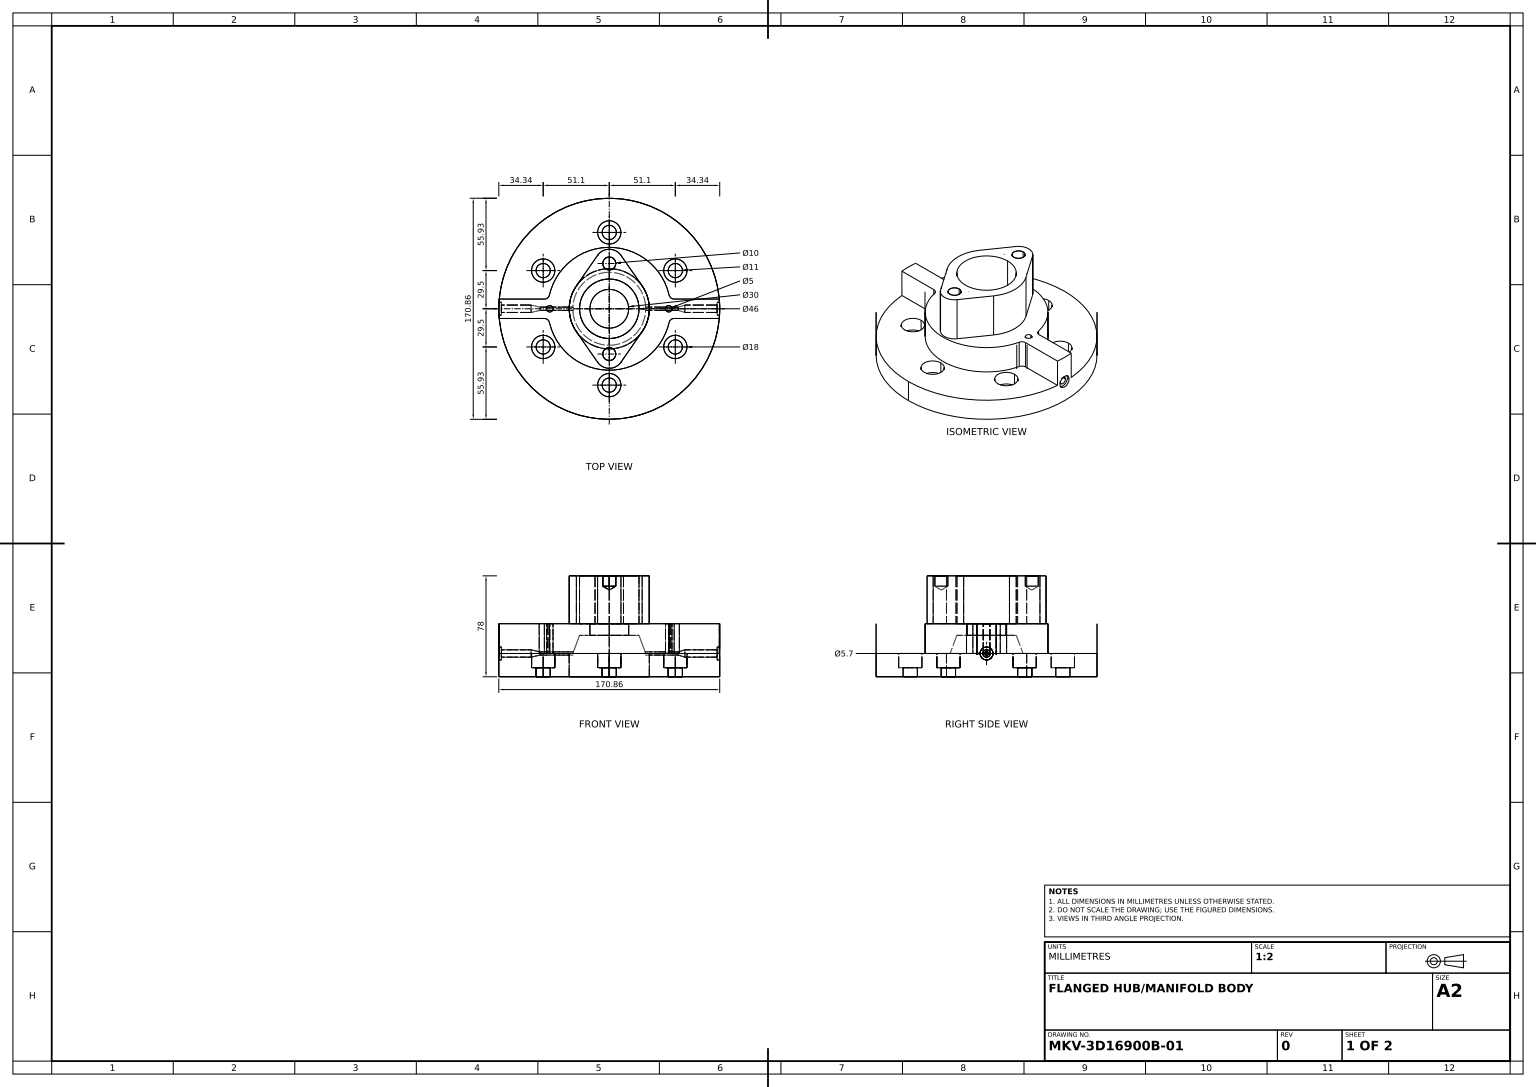
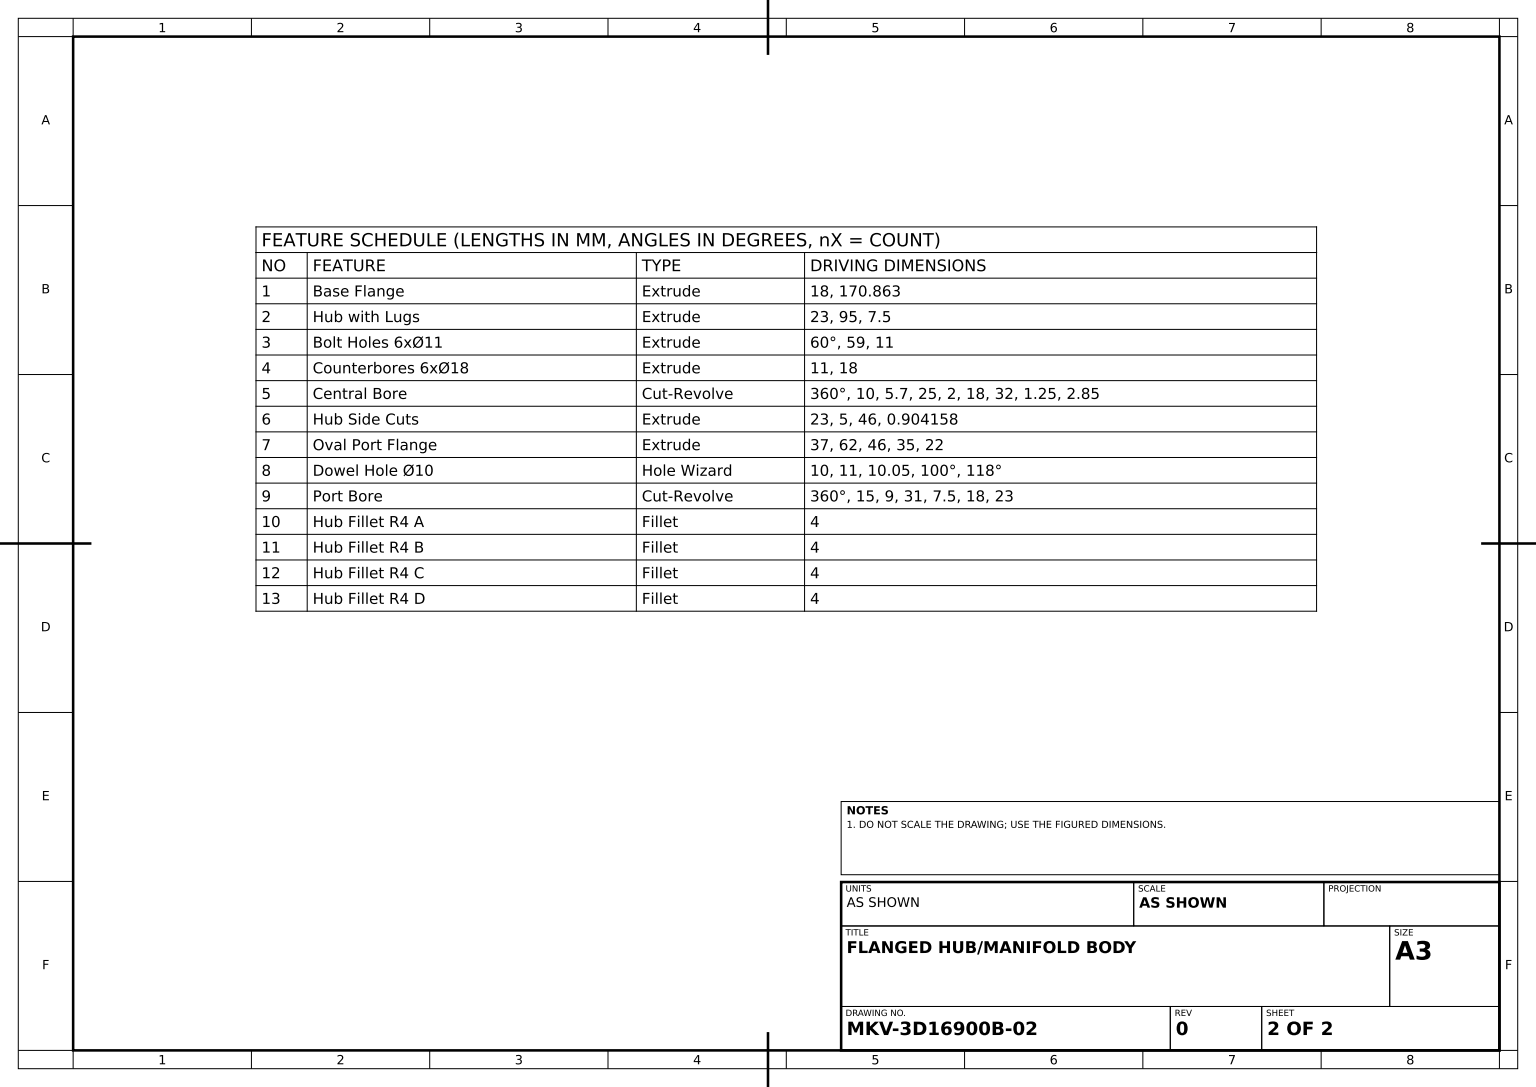
from build123d import *

# Parameters (mm, degrees)
BASE_FLANGE_SKETCH_R      = 85.431414023
BASE_FLANGE_DEPTH         = 18
HUB_WITH_LUGS_DEPTH       = 23
BOLT_HOLES_6X_11_REACH    = 124.988
BOLT_HOLES_SKETCH_R       = 5.5
COUNTERBORES_SKETCH_R     = 9
COUNTERBORES_6X_18_DEPTH  = 11
HUB_SIDE_CUTS_SKETCH_R    = 2.5
HUB_SIDE_CUTS_DEPTH       = 23
OVAL_PORT_FLANGE_SKETCH_R = 23
OVAL_PORT_FLANGE_DEPTH    = 37
DOWEL_HOLE_10_D           = 10
DOWEL_HOLE_10_DEPTH       = 7.995696905
DOWEL_HOLE_10_CSINK_D     = 10.05
DOWEL_HOLE_10_CSINK_ANGLE = 100
DOWEL_HOLE_10_TIP         = 3.004303095
HUB_FILLET_R4_A_R         = 4
HUB_FILLET_R4_B_R         = 4
HUB_FILLET_R4_C_R         = 4
HUB_FILLET_R4_D_R         = 4


with BuildPart() as part:
    # Base Flange Sketch → Base Flange (new body)
    with BuildSketch(Plane(origin=(0, 0, 0), x_dir=(1, 0, 0), z_dir=(0, 1, 0))):
        with Locations(Location((0, 0, 0), (0, 0, 270))):
            Circle(BASE_FLANGE_SKETCH_R)
    extrude(amount=BASE_FLANGE_DEPTH)

    # Hub with Lugs Sketch → Hub with Lugs (add)
    with BuildSketch(Plane(origin=(0, 18, 0), x_dir=(1, 0, 0), z_dir=(0, 1, 0))):
        with BuildLine():
            Line((-46.904157598, 7.5), (-85.101565802, 7.5))
            ThreePointArc((-85.101565802, 7.5), (-85.431414023, 0), (-85.101565802, -7.5))
            Line((-85.101565802, -7.5), (-46.904157598, -7.5))
            ThreePointArc((-46.904157598, -7.5), (0, -47.5), (46.904157598, -7.5))
            Line((46.904157598, -7.5), (85.101565802, -7.5))
            ThreePointArc((85.101565802, -7.5), (85.431414023, 0), (85.101565802, 7.5))
            Line((85.101565802, 7.5), (46.904157598, 7.5))
            ThreePointArc((46.904157598, 7.5), (0, 47.5), (-46.904157598, 7.5))
        make_face()
    extrude(amount=HUB_WITH_LUGS_DEPTH)

    # Bolt Holes Sketch → Bolt Holes 6xØ11 (cut, up to next)
    with BuildSketch(Plane(origin=(0, 18, 0), x_dir=(1, 0, 0), z_dir=(0, 1, 0)), mode=Mode.PRIVATE) as bolt_holes_6x_11_sk1:
        with Locations(Location((0, 59, 0), (0, 0, 270))):
            Circle(BOLT_HOLES_SKETCH_R)
    bolt_holes_6x_11_tool1 = extrude(bolt_holes_6x_11_sk1.sketch, amount=-BOLT_HOLES_6X_11_REACH, mode=Mode.PRIVATE) & part.part
    # Bolt Holes Sketch → Bolt Holes 6xØ11 (cut, up to next)
    with BuildSketch(Plane(origin=(0, 18, 0), x_dir=(1, 0, 0), z_dir=(0, 1, 0)), mode=Mode.PRIVATE) as bolt_holes_6x_11_sk2:
        with Locations(Location((0, -59, 0), (0, 0, 270))):
            Circle(BOLT_HOLES_SKETCH_R)
    bolt_holes_6x_11_tool2 = extrude(bolt_holes_6x_11_sk2.sketch, amount=-BOLT_HOLES_6X_11_REACH, mode=Mode.PRIVATE) & part.part
    # Bolt Holes Sketch → Bolt Holes 6xØ11 (cut, up to next)
    with BuildSketch(Plane(origin=(0, 18, 0), x_dir=(1, 0, 0), z_dir=(0, 1, 0)), mode=Mode.PRIVATE) as bolt_holes_6x_11_sk3:
        with Locations(Location((51.095498823, 29.5, 0), (0, 0, 270))):
            Circle(BOLT_HOLES_SKETCH_R)
    bolt_holes_6x_11_tool3 = extrude(bolt_holes_6x_11_sk3.sketch, amount=-BOLT_HOLES_6X_11_REACH, mode=Mode.PRIVATE) & part.part
    # Bolt Holes Sketch → Bolt Holes 6xØ11 (cut, up to next)
    with BuildSketch(Plane(origin=(0, 18, 0), x_dir=(1, 0, 0), z_dir=(0, 1, 0)), mode=Mode.PRIVATE) as bolt_holes_6x_11_sk4:
        with Locations(Location((51.095498823, -29.5, 0), (0, 0, 270))):
            Circle(BOLT_HOLES_SKETCH_R)
    bolt_holes_6x_11_tool4 = extrude(bolt_holes_6x_11_sk4.sketch, amount=-BOLT_HOLES_6X_11_REACH, mode=Mode.PRIVATE) & part.part
    # Bolt Holes Sketch → Bolt Holes 6xØ11 (cut, up to next)
    with BuildSketch(Plane(origin=(0, 18, 0), x_dir=(1, 0, 0), z_dir=(0, 1, 0)), mode=Mode.PRIVATE) as bolt_holes_6x_11_sk5:
        with Locations(Location((-51.095498823, -29.5, 0), (0, 0, 270))):
            Circle(BOLT_HOLES_SKETCH_R)
    bolt_holes_6x_11_tool5 = extrude(bolt_holes_6x_11_sk5.sketch, amount=-BOLT_HOLES_6X_11_REACH, mode=Mode.PRIVATE) & part.part
    # Bolt Holes Sketch → Bolt Holes 6xØ11 (cut, up to next)
    with BuildSketch(Plane(origin=(0, 18, 0), x_dir=(1, 0, 0), z_dir=(0, 1, 0)), mode=Mode.PRIVATE) as bolt_holes_6x_11_sk6:
        with Locations(Location((-51.095498823, 29.5, 0), (0, 0, 270))):
            Circle(BOLT_HOLES_SKETCH_R)
    bolt_holes_6x_11_tool6 = extrude(bolt_holes_6x_11_sk6.sketch, amount=-BOLT_HOLES_6X_11_REACH, mode=Mode.PRIVATE) & part.part
    add(bolt_holes_6x_11_tool1.solids().sort_by_distance((0, 18, -59))[0], mode=Mode.SUBTRACT)
    add(bolt_holes_6x_11_tool2.solids().sort_by_distance((0, 18, 59))[0], mode=Mode.SUBTRACT)
    add(bolt_holes_6x_11_tool3.solids().sort_by_distance((51.095499, 18, -29.5))[0], mode=Mode.SUBTRACT)
    add(bolt_holes_6x_11_tool4.solids().sort_by_distance((51.095499, 18, 29.5))[0], mode=Mode.SUBTRACT)
    add(bolt_holes_6x_11_tool5.solids().sort_by_distance((-51.095499, 18, 29.5))[0], mode=Mode.SUBTRACT)
    add(bolt_holes_6x_11_tool6.solids().sort_by_distance((-51.095499, 18, -29.5))[0], mode=Mode.SUBTRACT)

    # Counterbores Sketch → Counterbores 6xØ18 (cut)
    with BuildSketch(Plane(origin=(0, 18, 0), x_dir=(1, 0, 0), z_dir=(0, 1, 0))):
        with Locations(Location((0, 59, 0), (0, 0, 270))):
            Circle(COUNTERBORES_SKETCH_R)
        with Locations(Location((51.095498823, 29.5, 0), (0, 0, 270))):
            Circle(COUNTERBORES_SKETCH_R)
        with Locations(Location((51.095498823, -29.5, 0), (0, 0, 270))):
            Circle(COUNTERBORES_SKETCH_R)
        with Locations(Location((0, -59, 0), (0, 0, 270))):
            Circle(COUNTERBORES_SKETCH_R)
        with Locations(Location((-51.095498823, -29.5, 0), (0, 0, 270))):
            Circle(COUNTERBORES_SKETCH_R)
        with Locations(Location((-51.095498823, 29.5, 0), (0, 0, 270))):
            Circle(COUNTERBORES_SKETCH_R)
    extrude(amount=-COUNTERBORES_6X_18_DEPTH, mode=Mode.SUBTRACT)

    # Central Bore Profile → Central Bore (revolve, cut)
    with BuildSketch(Plane.XY, mode=Mode.PRIVATE) as central_bore_sk:
        Polygon((-85.431414023, 18), (-85.431414023, 23), (-83.431414023, 23), (-83.431414023, 20.85), (-60.431414023, 20.85), (-53.431414023, 19.25), (53.431414023, 19.25), (58.431414023, 20.85), (83.431414023, 20.85), (83.431414023, 23), (85.431414023, 23), (85.431414023, 18), align=None)
    revolve(central_bore_sk.sketch.rotate(Axis((-85.431414023, 18, 0), (1, 0, 0)), 90), axis=Axis((-85.431414023, 18, 0), (1, 0, 0)), mode=Mode.SUBTRACT)

    # Hub Side Cuts Sketch → Hub Side Cuts (cut)
    with BuildSketch(Plane(origin=(0, 41, 0), x_dir=(1, 0, 0), z_dir=(0, 1, 0))):
        with Locations(Location((46, 0, 0), (0, 0, 270))):
            Circle(HUB_SIDE_CUTS_SKETCH_R)
        with Locations(Location((-46, 0, 0), (0, 0, 270))):
            Circle(HUB_SIDE_CUTS_SKETCH_R)
    extrude(amount=-HUB_SIDE_CUTS_DEPTH, mode=Mode.SUBTRACT)

    # Oval Port Flange Sketch → Oval Port Flange (add)
    with BuildSketch(Plane(origin=(0, 41, 0), x_dir=(1, 0, 0), z_dir=(0, 1, 0))):
        with BuildLine():
            Line((-9.027169873, 41.285714286), (-25.440206006, 17.714285714))
            ThreePointArc((-25.440206006, 17.714285714), (-31, 0), (-25.440206006, -17.714285714))
            Line((-25.440206006, -17.714285714), (-9.027169873, -41.285714286))
            ThreePointArc((-9.027169873, -41.285714286), (0, -46), (9.027169873, -41.285714286))
            Line((9.027169873, -41.285714286), (25.440206006, -17.714285714))
            ThreePointArc((25.440206006, -17.714285714), (31, 0), (25.440206006, 17.714285714))
            Line((25.440206006, 17.714285714), (9.027169873, 41.285714286))
            ThreePointArc((9.027169873, 41.285714286), (0, 46), (-9.027169873, 41.285714286))
        make_face()
        with Locations(Location((0, 0, 0), (0, 0, 270))):
            Circle(OVAL_PORT_FLANGE_SKETCH_R, mode=Mode.SUBTRACT)
    extrude(amount=OVAL_PORT_FLANGE_DEPTH)

    # Dowel Hole Ø10
    with Locations(Plane(origin=(0, 78, 0), x_dir=(1, 0, 0), z_dir=(0, 1, 0))):
        with Locations((0, 35), (0, -35)):
            CounterSinkHole(DOWEL_HOLE_10_D / 2, DOWEL_HOLE_10_CSINK_D / 2, depth=DOWEL_HOLE_10_DEPTH, counter_sink_angle=DOWEL_HOLE_10_CSINK_ANGLE)
            with Locations((0, 0, -(DOWEL_HOLE_10_DEPTH + DOWEL_HOLE_10_TIP / 2))):  # 118° drill point
                Cone(0, DOWEL_HOLE_10_D / 2, DOWEL_HOLE_10_TIP, mode=Mode.SUBTRACT)

    # Port Bore Profile → Port Bore (revolve, cut)
    with BuildSketch(Plane.XY, mode=Mode.PRIVATE) as port_bore_sk:
        Polygon((-28.196580072, 18), (-31, 18), (-31, 0), (0, 0), (0, 41), (-15, 41), (-15, 32), (-23, 32), align=None)
    revolve(port_bore_sk.sketch.rotate(Axis((0, 78, 0), (0, -1, 0)), 270), axis=Axis((0, 78, 0), (0, -1, 0)), mode=Mode.SUBTRACT)

    # Hub Fillet R4 A
    hub_fillet_r4_a_edges = [part.edges().sort_by_distance(p)[0] for p in [
        (46.904157598, 29.5, 7.5),
    ]]
    fillet(hub_fillet_r4_a_edges, radius=HUB_FILLET_R4_A_R)

    # Hub Fillet R4 B
    hub_fillet_r4_b_edges = [part.edges().sort_by_distance(p)[0] for p in [
        (46.904157598, 29.5, -7.5),
    ]]
    fillet(hub_fillet_r4_b_edges, radius=HUB_FILLET_R4_B_R)

    # Hub Fillet R4 C
    hub_fillet_r4_c_edges = [part.edges().sort_by_distance(p)[0] for p in [
        (-46.904157598, 29.5, -7.5),
    ]]
    fillet(hub_fillet_r4_c_edges, radius=HUB_FILLET_R4_C_R)

    # Hub Fillet R4 D
    hub_fillet_r4_d_edges = [part.edges().sort_by_distance(p)[0] for p in [
        (-46.904157598, 29.5, 7.5),
    ]]
    fillet(hub_fillet_r4_d_edges, radius=HUB_FILLET_R4_D_R)


solid = part.part
